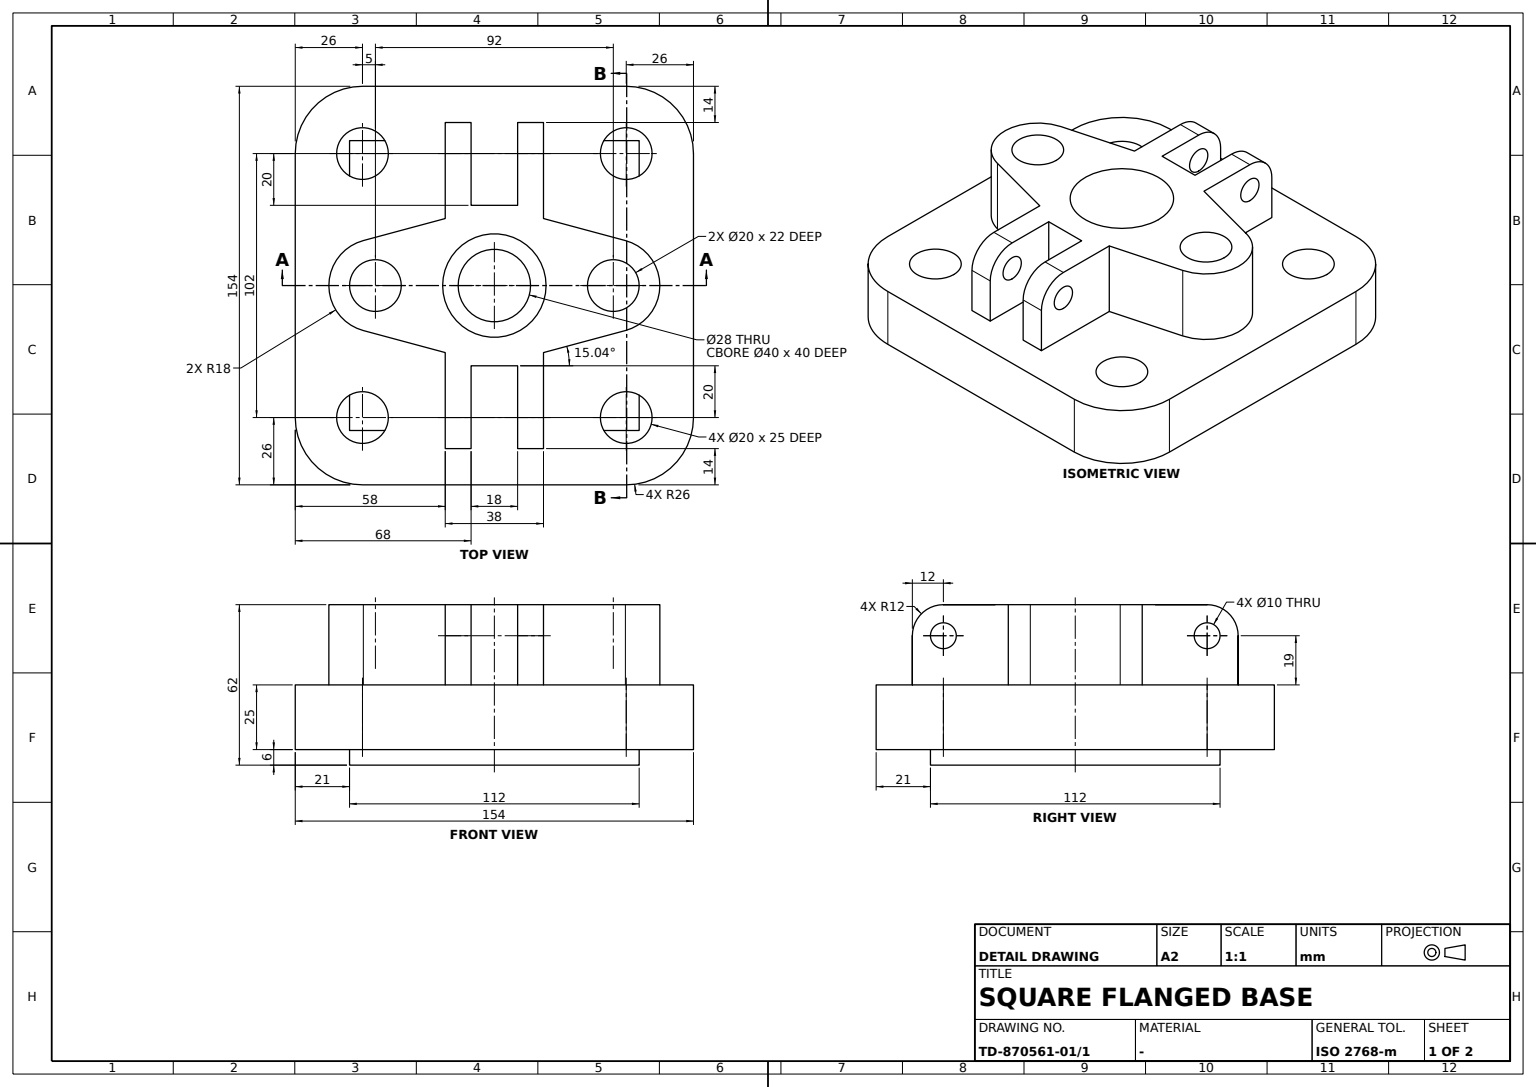
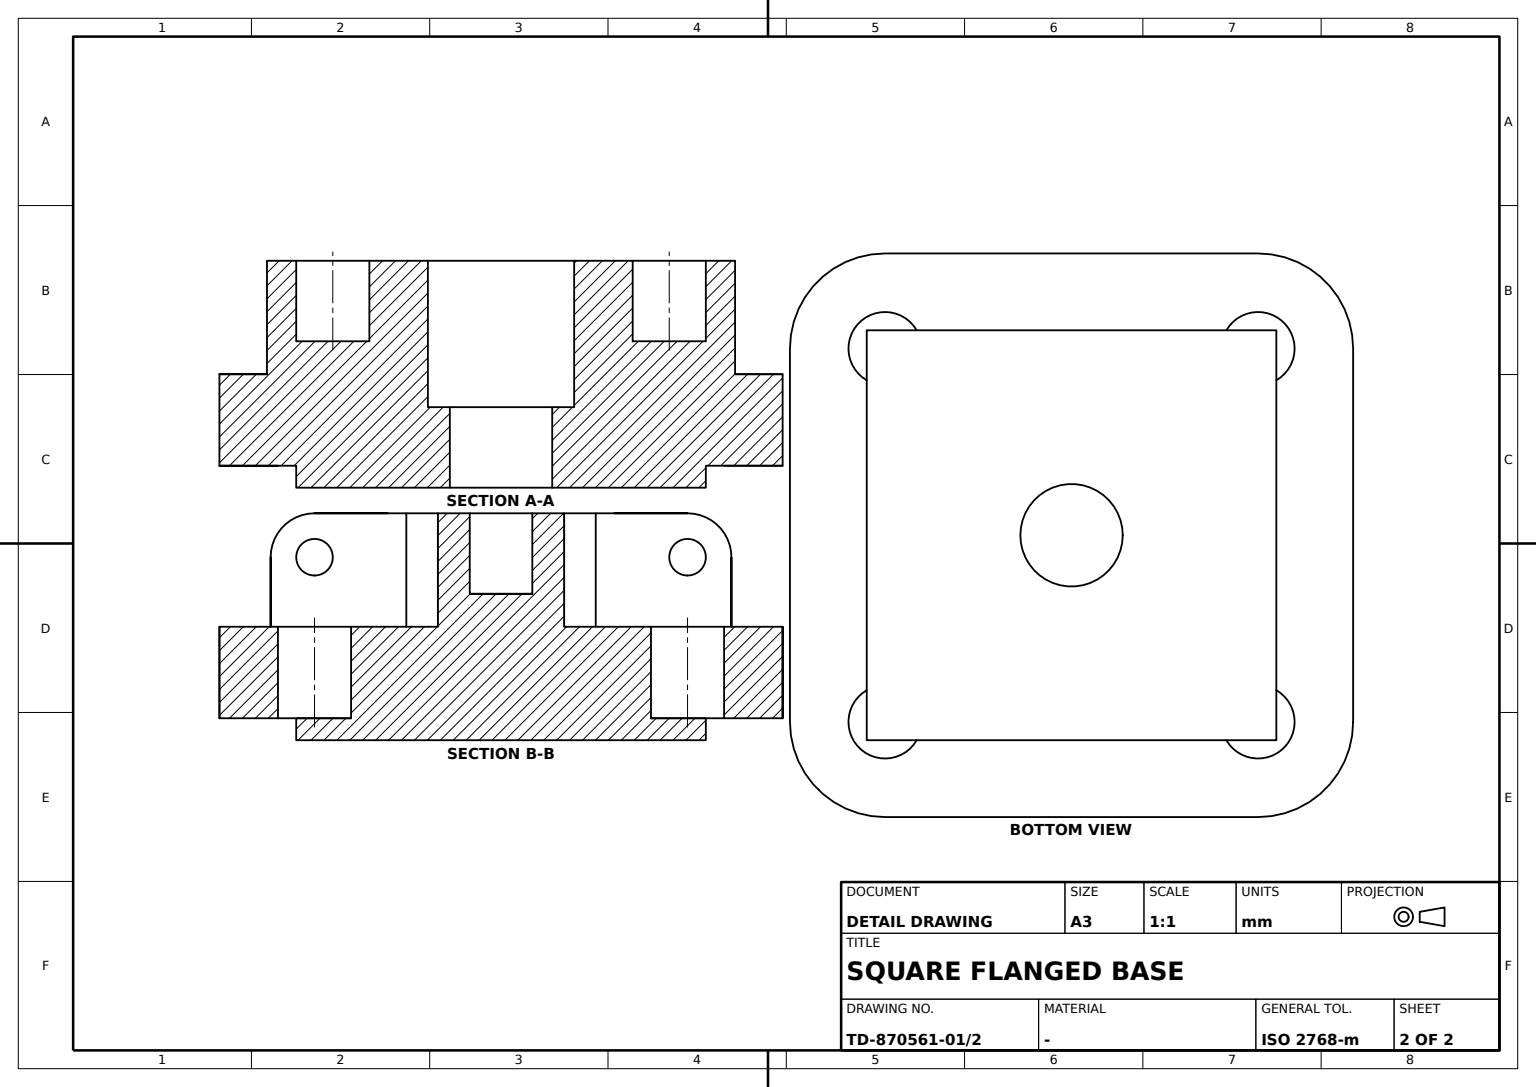
CATIA V5 part; units mm, degrees
sketch "Sketch1" plane through (0, 0, 0) normal (0, 0, 1) x (1, 0, 0)
  line L0 (77, 51) -> (77, -51)
  line L1 (51, -77) -> (-51, -77)
  line L2 (-77, -51) -> (-77, 51)
  line L3 (-51, 77) -> (51, 77)
  point P0 (77, 77)
  point P1 (77, -77)
  point P2 (-77, 77)
  arc A0 (-77, 51) -> (-51, 77) centre (-51, 51) cw
  arc A1 (77, 51) -> (51, 77) centre (51, 51) ccw
  arc A2 (-51, -77) -> (-77, -51) centre (-51, -51) cw
  arc A3 (77, -51) -> (51, -77) centre (51, -51) cw
  dimension "distance P2 P0" = 154
  dimension "radius A0" = 26
  dimension "distance P0 P1" = 154
  dimension "radius A1" = 26
  dimension "radius A2" = 26
  dimension "radius A3" = 26
  constraint vertical L0 y-axis
  constraint vertical L2 y-axis
  constraint horizontal L1 x-axis
  constraint horizontal L3 x-axis
  constraint equidistance L0 L2 origin
  constraint equidistance L1 L3 origin
  constraint coincidence L2 P2
  constraint coincidence L3 P2
  constraint coincidence L0 P0
  constraint coincidence L3 P0
  constraint coincidence L0 P1
  constraint coincidence L1 P1
  constraint tangency A0 L2
  constraint tangency A0 L3
  constraint tangency A1 L0
  constraint tangency A1 L3
  constraint tangency A2 L1
  constraint tangency A2 L2
  constraint tangency A3 L0
  constraint tangency A3 L1
extrude "Pad1" add sketch "Sketch1" along normal blind 25
sketch "Sketch2" plane through (0, 0, 0) normal (0, 0, 1) x (1, 0, 0)
  circle A0 centre (-51, 51) radius 10
  circle A1 centre (51, 51) radius 10
  circle A2 centre (-51, -51) radius 10
  circle A3 centre (51, -51) radius 10
  arc A4 (51, -77) -> (77, -51) centre (51, -51) ccw construction
  arc A5 (77, 51) -> (51, 77) centre (51, 51) ccw construction
  arc A6 (-51, 77) -> (-77, 51) centre (-51, 51) ccw construction
  arc A7 (-77, -51) -> (-51, -77) centre (-51, -51) ccw construction
  dimension "radius A0" = 10
  dimension "radius A1" = 10
  dimension "radius A3" = 10
  dimension "radius A2" = 10
  constraint concentricity A3 A4
  constraint concentricity A1 A5
  constraint concentricity A0 A6
  constraint concentricity A2 A7
extrude "Pocket1" cut sketch "Sketch2" along normal blind 25
sketch "Sketch3" plane through (0, 0, 0) normal (0, 0, 1) x (1, 0, 0)
  line L0 (-46, 0) -> (46, 0) construction
  point P0 (-46, 0)
  point P1 (46, 0)
  line L1 (0, 31) -> (0, -31) construction
  point P2 (0, 31)
  point P3 (0, -31)
  arc A0 (-50.6713, 17.3833) -> (-50.6713, -17.3833) centre (-46, 0) ccw
  line L2 (-19, 25.8942) -> (-50.6713, 17.3833)
  line L3 (-19, -25.8942) -> (-50.6713, -17.3833)
  point P4 (-50.6713, 17.3833)
  point P5 (-50.6713, -17.3833)
  point P6 (-50.6713, 17.3833)
  point P7 (50.6713, 17.3833)
  line L4 (19, 25.8942) -> (50.6713, 17.3833)
  point P8 (50.6713, -17.3833)
  point P9 (50.6713, 17.3833)
  arc A1 (50.6713, 17.3833) -> (50.6713, -17.3833) centre (46, 0) cw
  line L5 (19, -25.8942) -> (50.6713, -17.3833)
  point P10 (-19, 0)
  line L6 (-19, 25.8942) -> (-19, 63)
  point P11 (-19, 63)
  line L7 (-19, 63) -> (-9, 63)
  point P12 (-9, 63)
  line L8 (-9, 63) -> (-9, 31)
  point P13 (-9, 31)
  line L9 (-9, 31) -> (9, 31)
  point P14 (9, 31)
  line L10 (9, 31) -> (9, 63)
  point P15 (9, 63)
  line L11 (9, 63) -> (19, 63)
  point P16 (19, 63)
  line L12 (19, 63) -> (19, 25.8942)
  point P17 (19, 0)
  line L13 (51, 77) -> (-51, 77) construction
  point P18 (-19, -63)
  line L14 (-19, -25.8942) -> (-19, -63)
  point P19 (-9, -63)
  line L15 (-19, -63) -> (-9, -63)
  point P20 (-9, -31)
  line L16 (-9, -63) -> (-9, -31)
  point P21 (9, -63)
  point P22 (9, -31)
  line L17 (9, -31) -> (9, -63)
  point P23 (19, -63)
  line L18 (9, -63) -> (19, -63)
  line L19 (19, -63) -> (19, -25.8942)
  line L20 (-9, -31) -> (9, -31)
  dimension "length L0" = 92
  dimension "length L1" = 62
  dimension "radius A0" = 18
  dimension "length L7" = 10
  dimension "length L9" = 18
  dimension "distance L13 L7" = 14
  dimension "distance L9 P2" = 0
  constraint coincidence P0 x-axis
  constraint coincidence P2 y-axis
  constraint coincidence A0 P4
  constraint coincidence L2 P6
  constraint coincidence P10 L0
  constraint coincidence P15 L7
  constraint coincidence P17 L0
  constraint coincidence P4 P6
  constraint coincidence P7 P9
  constraint horizontal L0 x-axis
  constraint horizontal L7 x-axis
  constraint horizontal L9 x-axis
  constraint horizontal L11 x-axis
  constraint symmetry P1 P0 y-axis
  constraint symmetry P2 P3 x-axis
  constraint symmetry P4 P7 y-axis
  constraint symmetry L2 L4 y-axis
  constraint symmetry P5 P8 y-axis
  constraint symmetry P6 P9 y-axis
  constraint symmetry A0 A1 y-axis
  constraint symmetry L3 L5 y-axis
  constraint symmetry L6 L12 y-axis
  constraint symmetry L8 L10 y-axis
  constraint symmetry P11 P18 x-axis
  constraint symmetry L6 L14 x-axis
  constraint symmetry P12 P19 x-axis
  constraint symmetry L7 L15 x-axis
  constraint symmetry P13 P20 x-axis
  constraint symmetry L8 L16 x-axis
  constraint symmetry P15 P21 x-axis
  constraint symmetry P14 P22 x-axis
  constraint symmetry L10 L17 x-axis
  constraint symmetry P16 P23 x-axis
  constraint symmetry L11 L18 x-axis
  constraint symmetry L12 L19 x-axis
  constraint symmetry L9 L20 x-axis
  constraint vertical L1 y-axis
  constraint vertical L6 y-axis
  constraint vertical L8 y-axis
  constraint vertical L10 y-axis
  constraint vertical L12 y-axis
  constraint tangency L2 A0
  constraint tangency L3 A0
extrude "Pad2" add sketch "Sketch3" along normal blind 56
fillet "Fillet1" radius 12 4 edges at (14, 63, 56) (-14, 63, 56) (-14, -63, 56) (14, -63, 56)
sketch "Sketch4" plane through (0, 0, 0) normal (1, 0, 0) x (0, 1, 0)
  circle A0 centre (51, 44) radius 5
  arc A1 (63, 44) -> (51, 56) centre (51, 44) ccw construction
  circle A2 centre (-51, 44) radius 5
  dimension "radius A0" = 5
  constraint concentricity A0 A1
  constraint symmetry A0 A2 y-axis
extrude "Pocket2" cut sketch "Sketch4" along normal mid plane 112
sketch "Sketch6" plane through (0, 0, 0) normal (0, 0, 1) x (1, 0, 0)
  line L0 (56, 56) -> (56, -56)
  line L1 (56, -56) -> (-56, -56)
  line L2 (-56, -56) -> (-56, 56)
  line L3 (-56, 56) -> (56, 56)
  dimension "length L3" = 112
  dimension "length L0" = 112
  constraint vertical L0 y-axis
  constraint vertical L2 y-axis
  constraint horizontal L1 x-axis
  constraint horizontal L3 x-axis
  constraint equidistance L0 L2 origin
  constraint equidistance L1 L3 origin
extrude "Pad3" add sketch "Sketch6" against normal blind 6
sketch "Sketch5" plane through (0, 0, 56) normal (0, 0, 1) x (1, 0, 0)
  circle A0 centre (0, 0) radius 14
  circle A1 centre (0, 0) radius 20
  dimension "radius A1" = 20
  dimension "radius A0" = 14
extrude "MultiPocket1 domain 1" cut sketch "Sketch5" against normal blind 40 contours A1
extrude "MultiPocket1 domain 2" cut sketch "Sketch5" against normal blind 62 contours A0
sketch "Sketch7" plane through (0, 0, 56) normal (0, 0, 1) x (1, 0, 0)
  circle A0 centre (46, 0) radius 10
  point P0 (46, 0)
  arc A1 (50.6713, -17.3833) -> (50.6713, 17.3833) centre (46, 0) ccw construction
  circle A2 centre (-46, 0) radius 10
  dimension "radius A0" = 10
  constraint coincidence P0 x-axis
  constraint concentricity A0 A1
  constraint symmetry A0 A2 y-axis
extrude "Pocket3" cut sketch "Sketch7" against normal blind 22
properties part number "22"
